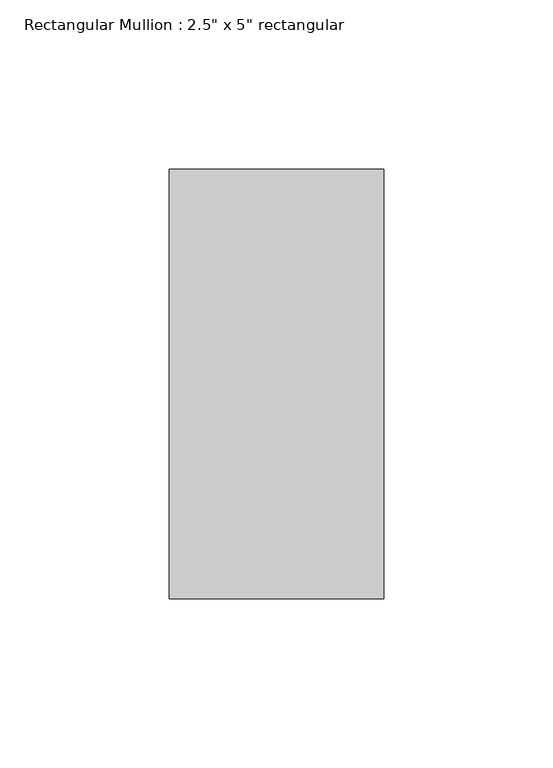
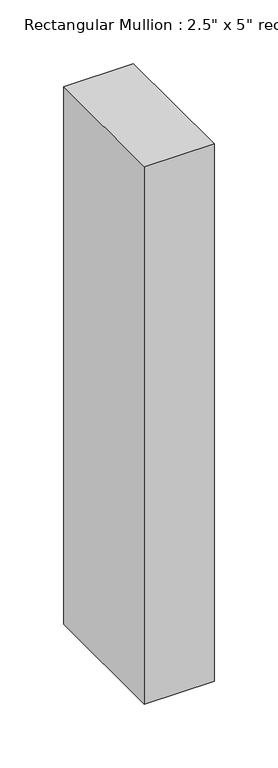
"""IFC4 building model written with IfcOpenShell, lengths in millimetres: member geometry."""

from ifc_helpers import new_model, si_unit, frame, origin, place, context, project, spatial, polyline, outline, extrude, source, transform, mapped, element, save


def member_ce4f90f2(model_context):
    return source(origin(), model_context, "Body", "SweptSolid", [
        extrude(outline(polyline([(0.0, 63.5), (0.0, -63.5), (-63.5, -63.5), (-63.5, 63.5), (0.0, 63.5)])), frame((0.0, 0.0, -516.4666667), z_axis=(0.0, 0.0, 1.0), x_axis=(1.0, 0.0, 0.0)), (0.0, 0.0, 1.0), 516.4666667),
    ])


if __name__ == "__main__":
    model = new_model("IFC4")
    model_context = context("Model", 3, world=origin())
    ifc_project = project(units=[si_unit("LENGTHUNIT", "METRE", prefix="MILLI")], contexts=[model_context])
    site = spatial("IfcSite", under=ifc_project)
    building = spatial("IfcBuilding", under=site)
    placement = place(None, origin())
    member_shape = member_ce4f90f2(model_context)
    element("IfcMember", 1, ObjectType="Rectangular Mullion : 2.5\" x 5\" rectangular", at=placement, inside=building, context=model_context, shape_type="MappedRepresentation", body=[
        mapped(member_shape, transform((0.0, 0.0, 0.0), x_axis=(1.0, 0.0, 0.0), y_axis=(0.0, 1.0, 0.0), z_axis=(0.0, 0.0, 1.0))),
    ])
    save(model, "model.ifc")

# Revit data of these elements
# Type "Rectangular Mullion : 2.5\" x 5\" rectangular"
#   built-in parameter 1007304 = 0.416667 (stored number, unit not read)
#   built-in parameter 1007301 = 0.104167 (stored number, unit not read)
#   built-in parameter 1007300 = 0.104167 (stored number, unit not read)
